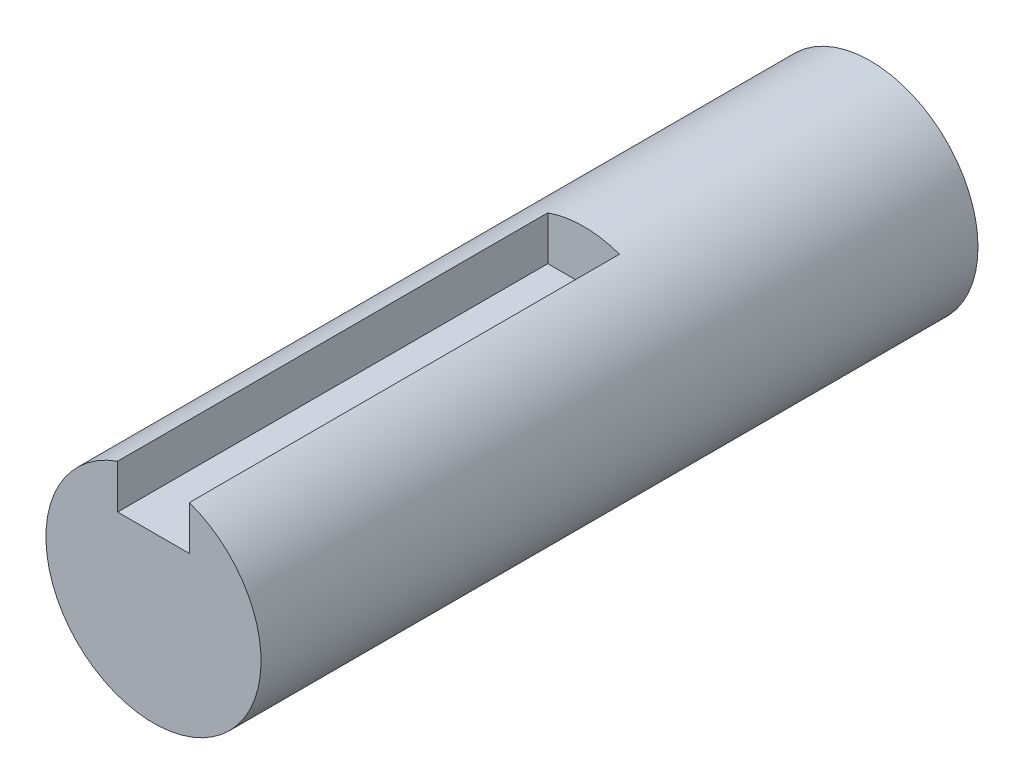
from build123d import *

# Parameters (mm, degrees)
SHAFT_PROFILE_30_R      = 15
SHAFT_BODY_30X100_DEPTH = 100
KEYWAY_PROFILE_W        = 10
KEYWAY_PROFILE_H        = 7
KEYWAY_CUT_60MM_DEPTH   = 60


with BuildPart() as part:
    # Shaft Profile Ø30 → Shaft Body Ø30x100 (new body)
    with BuildSketch(Plane.XY):
        Circle(SHAFT_PROFILE_30_R)
    extrude(amount=SHAFT_BODY_30X100_DEPTH)

    # Keyway Profile → Keyway Cut 60mm (cut)
    with BuildSketch(Plane.XY.offset(100)):
        with Locations((0, 11.5)):
            Rectangle(KEYWAY_PROFILE_W, KEYWAY_PROFILE_H)
    extrude(amount=-KEYWAY_CUT_60MM_DEPTH, mode=Mode.SUBTRACT)


solid = part.part
